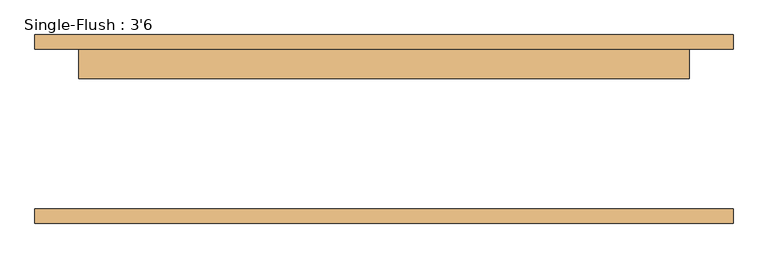
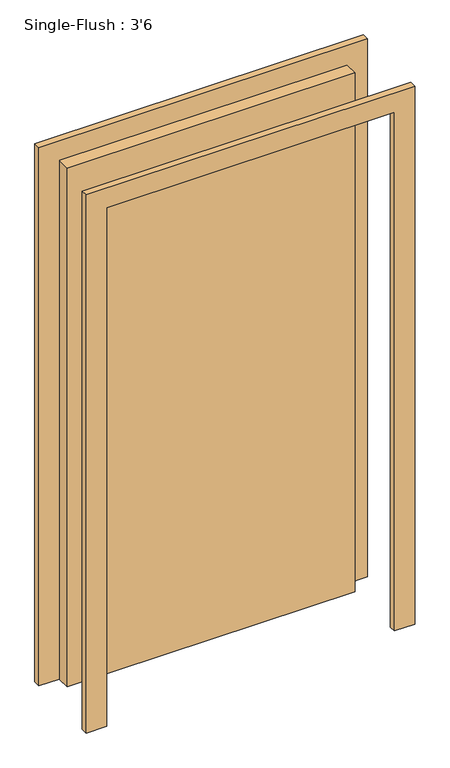
"""IFC4 building model written with IfcOpenShell, lengths in millimetres: door geometry, Single-Flush : 3'6."""

from ifc_helpers import new_model, si_unit, frame, origin, origin_with_axes, place, context, project, spatial, polyline, outline, extrude, source, transform, mapped, element, save


def single_flush_3_6_472124c4(model_context):
    return source(origin(), model_context, "Body", "SweptSolid", [
        extrude(outline(polyline([(2108.2, -609.6), (0.0, -609.6), (0.0, -533.4), (2032.0, -533.4), (2032.0, 533.4), (0.0, 533.4), (0.0, 609.6), (2108.2, 609.6), (2108.2, -609.6)])), frame((0.0, 139.7, 0.0), z_axis=(0.0, 1.0, 0.0), x_axis=(0.0, 0.0, 1.0)), (0.0, 0.0, 1.0), 25.4),
        extrude(outline(polyline([(2108.2, 609.6), (2108.2, -609.6), (0.0, -609.6), (0.0, -533.4), (2032.0, -533.4), (2032.0, 533.4), (0.0, 533.4), (0.0, 609.6), (2108.2, 609.6)])), frame((0.0, -165.1, 0.0), z_axis=(0.0, 1.0, 0.0), x_axis=(0.0, 0.0, 1.0)), (0.0, 0.0, 1.0), 25.4),
        extrude(outline(polyline([(533.4, 88.9), (-533.4, 88.9), (-533.4, 139.7), (533.4, 139.7), (533.4, 88.9)])), origin_with_axes(), (0.0, 0.0, 1.0), 2032.0),
    ])


if __name__ == "__main__":
    model = new_model("IFC4")
    model_context = context("Model", 3, world=origin())
    ifc_project = project(units=[si_unit("LENGTHUNIT", "METRE", prefix="MILLI")], contexts=[model_context])
    site = spatial("IfcSite", under=ifc_project)
    building = spatial("IfcBuilding", under=site)
    placement = place(None, origin())
    single_flush_3_6_shape = single_flush_3_6_472124c4(model_context)
    element("IfcDoor", 1, ObjectType="Single-Flush : 3'6", at=placement, inside=building, context=model_context, shape_type="MappedRepresentation", body=[
        mapped(single_flush_3_6_shape, transform((0.0, 0.0, 0.0), x_axis=(1.0, 0.0, 0.0), y_axis=(0.0, 1.0, 0.0), z_axis=(0.0, 0.0, 1.0))),
    ])
    save(model, "model.ifc")

# Revit data of these elements
# Type "Single-Flush : 3'6"
#   Type Mark = "8"
#   Construction Type Id = "MDOOR"
#   Assembly Code = "C1020"
#   Analytic Construction = "Metal"
#   Thickness = 2"
#   Heat Transfer Coefficient (U) = 0.651978 BTU/(h·ft²·°F)
#   Height = 80"
#   Trim Projection Ext = 1"
#   Trim Projection Int = 1"
#   Trim Width = 3"
#   Width = 42"
#   Define Thermal Properties by = 1
#   Door Material = Door - Panel
#   Frame Material = Door - Frame
#   Visual Light Transmittance = 0
#   Solar Heat Gain Coefficient = 0
#   Function = (empty or 0)
#   Wall Closure = (empty or 0)
# Element 1 (IfcDoor, "Single-Flush : 3'6")
#   Materials on its faces: "Door - Frame", "Door - Panel"
# Materials
#   "Door - Panel": class "Wood", colour RGB 210 159 95, transparency 0, Cost = 0
#   "Door - Frame": colour RGB 118 70 51, transparency 0, Cost = 0
